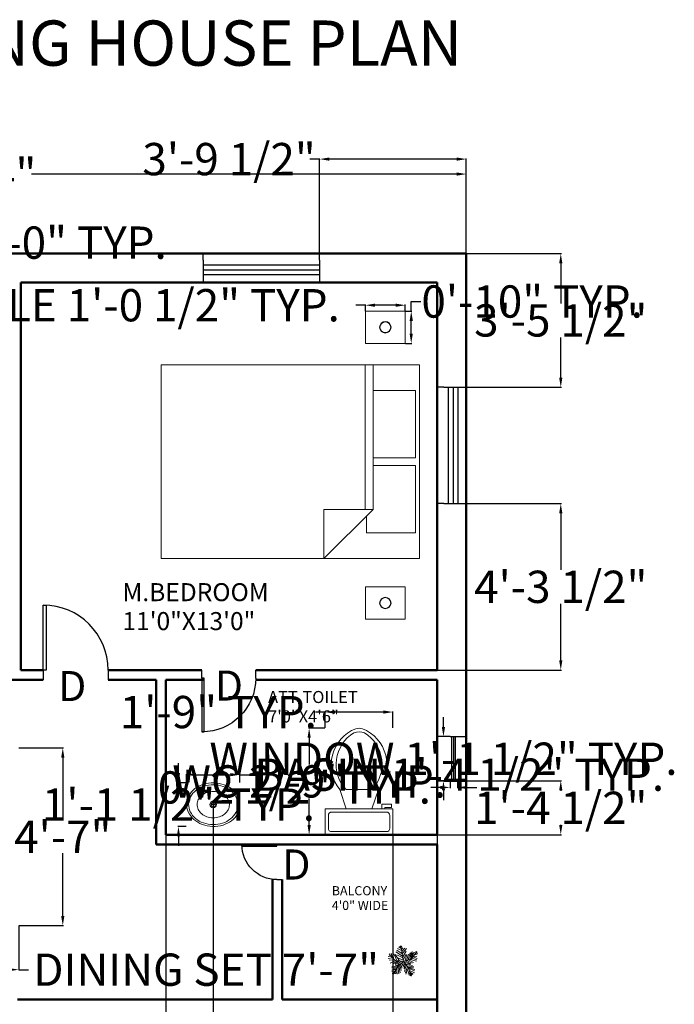
# Model space of a CAD drawing. Units: inches. Extents: x -35 to 382, y 867 to 1468.
# Tile 3 of 3: x 179 to 382, y 1163 to 1468. Entities that reach past the tile are written whole.
import ezdxf

# ---------------------------------------------------------------- set-up
doc = ezdxf.new("R2010")
doc.units = ezdxf.units.IN
doc.header["$MEASUREMENT"] = 0
for name, color, linetype, lineweight in [('A-ANNO-DIMS', 2, 'Continuous', 18), ('A-ANNO-TEXT', 7, 'Continuous', 25), ('A-AREA-IDEN', 7, 'Continuous', 25), ('A-DOOR', 3, 'Continuous', 25), ('A-FLOR-FIXT', 9, 'Continuous', 18), ('A-FURN', 9, 'Continuous', 18), ('A-GLAZ', 4, 'Continuous', 25), ('A-WALL', 7, 'Continuous', 50), ('L-PLNT', 94, 'Continuous', 13)]:
    doc.layers.add(name, color=color, linetype=linetype, lineweight=lineweight)
doc.styles.get("Standard").update_dxf_attribs({"font": 'arial.ttf'})
doc.dimstyles.get("Standard").update_dxf_attribs({"dimtxt": 10, "dimasz": 3, "dimexe": 0.18, "dimexo": 0.0625, "dimgap": 0.09, "dimtad": 0, "dimtih": 1, "dimtoh": 1, "dimdec": 0, "dimzin": 0, "dimdsep": 46, "dimlunit": 3, "dimtxsty": 'Standard', "dimcen": 0.09, "dimadec": 0, "dimazin": 0, "dimtfac": 1, "dimtdec": 0, "dimtofl": 0, "dimtmove": 0, "dimatfit": 3, "dimfxl": 1, "dimtolj": 1, "dimtzin": 0, "dimarcsym": 0})

# ---------------------------------------------------------------- blocks, each defined once
blk = doc.blocks.new('Bed - Queen')
for p, q in [((0, -80.00003), (0, 0)), ((0, 0), (59.99999, 0)), ((59.99999, 0), (59.99999, -80.00003)), ((7.99999, -1.2), (28.79998, -1.2)), ((7.99999, -14.4), (7.99999, -1.2)), ((28.79998, -1.2), (28.79998, -14.4)), ((31.19999, -1.2), (51.99999, -1.2)), ((31.19999, -14.4), (31.19999, -1.2)), ((51.99999, -1.2), (51.99999, -16.4)), ((0, -14.4), (44.8, -14.4)), ((59.99999, -29.6), (44.8, -14.4)), ((44.8, -14.4), (44.8, -29.6)), ((44.8, -16.8), (0, -16.8)), ((51.99999, -16.4), (46.79936, -16.4)), ((44.8, -29.6), (59.99999, -29.6)), ((59.99999, -80.00003), (0, -80.00003))]:
    blk.add_line(p, q)
blk = doc.blocks.new('Sink - Oval top')
for p, q in [((-1, 0), (1, 0)), ((0, 1), (0, -1))]:
    blk.add_line(p, q)
for points in [[(-12.23, 0.39, 0.117634), (-11.46, -3.36, 0.104469), (-8.88, -6.8, 0.090016), (-5.08, -9.07, 0.08192), (-0.32, -10.02, 0.08192), (4.49, -9.38, 0.090016), (8.42, -7.36, 0.104469), (11.22, -4.09, 0.117634), (12.23, -0.39, 0.117634), (11.46, 3.36, 0.104469), (8.88, 6.8, 0.090016), (5.08, 9.07, 0.08192), (0.32, 10.02, 0.08192), (-4.49, 9.38, 0.090016), (-8.42, 7.36, 0.104469), (-11.22, 4.09, 0.117634)], [(-11.29, 0.16, 0.118622), (-10.52, -3.25, 0.104678), (-8.07, -6.36, 0.089562), (-4.54, -8.37, 0.081185), (-0.13, -9.15, 0.081185), (4.3, -8.49, 0.089562), (7.89, -6.58, 0.104678), (10.42, -3.55, 0.118622), (11.29, -0.16, 0.118622), (10.52, 3.25, 0.104678), (8.07, 6.36, 0.089562), (4.54, 8.37, 0.081185), (0.13, 9.15, 0.081185), (-4.3, 8.49, 0.089562), (-7.89, 6.58, 0.104678), (-10.42, 3.55, 0.118622)], [(-7.42, 0.08, 0.118283), (-6.91, -2.17, 0.104607), (-5.29, -4.21, 0.089718), (-2.97, -5.53, 0.081436), (-0.07, -6.04, 0.081436), (2.84, -5.59, 0.089718), (5.2, -4.33, 0.104607), (6.86, -2.32, 0.118283), (7.42, -0.08, 0.118283), (6.91, 2.17, 0.104607), (5.29, 4.21, 0.089718), (2.97, 5.53, 0.081436), (0.07, 6.04, 0.081436), (-2.84, 5.59, 0.089718), (-5.2, 4.33, 0.104607), (-6.86, 2.32, 0.118283)]]:
    blk.add_lwpolyline(points, format="xyb", close=True)
for radius in [1.5, 1]:
    blk.add_circle((0, 0), radius)
blk = doc.blocks.new('*U13')
for p, q in [((-93.091, 489.5342), (-700.3796, 902.3858)), ((-129.8956, 713.6638), (-626.7704, 1032.1544)), ((-185.1152, 1008.5578), (-553.1612, 1185.4942)), ((-221.9198, 1197.3052), (-433.5526, 1338.8594)), ((-258.7244, 1362.456), (-332.3336, 1421.4348)), ((0, 0), (-266.7, 1447.8)), ((-231.1146, 1315.2628), (-166.7002, 1421.4348)), ((-194.31, 1102.9442), (-65.4812, 1256.284)), ((-148.3106, 914.1968), (118.5418, 1220.9018)), ((-129.8956, 701.8528), (265.7602, 1185.4942)), ((-74.7014, 418.7444), (219.7608, 961.39)), ((685.8, 228.6), (1219.2, 914.4)), ((689.0258, 230.0224), (790.2448, 914.1968)), ((1121.4862, 925.9824), (1149.0706, 831.6214)), ((-1206.4492, 501.3198), (-1418.082, 465.9376)), ((-1031.621, 347.98), (-1399.667, 277.1902)), ((-800.1, 114.3), (-1333.5, 647.7)), ((-847.598, 159.2326), (-1326.0578, 135.636)), ((-1234.059, 536.7274), (-1252.4486, 737.2604)), ((-718.7946, 88.4682), (-1215.644, -147.447)), ((-1105.2302, 725.4494), (-1077.6458, 395.1732)), ((-976.4268, 666.4706), (-884.4026, 194.6402)), ((-543.9664, 76.6572), (-967.2066, -206.4512)), ((-902.8176, 713.6638), (-617.5756, 100.2538)), ((0, 0), (-800.1, 114.3)), ((-369.1382, 53.086), (-783.1836, 642.874)), ((-405.9428, 53.086), (-764.794, -241.8334)), ((-617.5756, 607.4918), (-74.7014, 347.98)), ((0, 0), (-571.5, -495.3)), ((-166.7002, 29.4894), (-543.9664, -206.4512)), ((-525.5514, 347.98), (-28.6766, 123.8504)), ((-28.6766, 171.0436), (228.9556, 678.2816)), ((0, 0), (685.8, 228.6)), ((0, 0), (457.2, -571.5)), ((100.1268, 41.275), (284.1498, 619.2774)), ((164.5412, 41.275), (661.416, -218.2368)), ((256.5654, 88.4682), (449.7832, 666.4706)), ((284.1498, 88.4682), (781.0246, -147.447)), ((412.9786, 147.447), (587.8068, 796.2392)), ((458.978, 147.447), (891.4384, -88.4682)), ((560.197, 182.8292), (698.2206, 819.8358)), ((615.4166, 194.6402), (1185.8752, 41.275)), ((753.4148, 312.5978), (1222.6798, 159.2326)), ((808.6344, 784.4282), (827.0494, 418.7444)), ((845.439, 418.7444), (1241.0948, 277.1902)), ((891.4384, 831.6214), (946.658, 572.1096)), ((919.0482, 501.3198), (1222.6798, 454.152)), ((983.4626, 867.0036), (1066.2666, 725.4494)), ((1029.462, 654.685), (1241.0948, 631.0884)), ((1112.2914, 760.8316), (1296.3144, 784.4282)), ((-442.7474, -383.3876), (-1086.8406, -477.7486)), ((-718.7946, -737.2604), (-1086.8406, -796.2392)), ((-617.5756, -548.5384), (-1077.6458, -560.324)), ((-783.1836, -867.029), (-1077.6458, -902.4112)), ((-681.9646, -666.496), (-1022.4262, -654.685)), ((-571.5, -495.3), (-952.5, -1143)), ((-387.5278, -324.4088), (-764.794, -324.4088)), ((-737.1842, -784.4536), (-709.5744, -1114.7298)), ((-635.9652, -607.5172), (-580.771, -1150.1374)), ((-525.5514, -465.963), (-451.9422, -1126.5408)), ((-166.7002, -147.447), (-507.1618, -253.619)), ((-433.5526, -383.3876), (-323.1134, -1020.3688)), ((-341.5284, -289.0012), (-221.9198, -831.6214)), ((-240.3094, -218.2368), (-157.5054, -595.7062)), ((-120.7008, -88.4682), (-93.091, -371.5766)), ((63.3222, -76.6826), (-37.8714, -513.1308)), ((44.9326, -64.897), (615.4166, -241.8334)), ((127.7366, -159.258), (54.1274, -654.685)), ((228.9556, -289.0012), (90.932, -914.1968)), ((357.759, -430.5554), (164.5412, -1020.3688)), ((192.151, -230.0224), (817.8292, -371.5766)), ((458.978, -572.1096), (210.5406, -1161.923)), ((311.7596, -383.3876), (937.4378, -477.7486)), ((514.1976, -772.6426), (403.7838, -1138.3264)), ((412.9786, -501.3452), (919.0482, -583.9206)), ((457.2, -571.5), (685.8, -1333.5)), ((468.1982, -572.1096), (1029.462, -737.2604)), ((486.5878, -642.8994), (983.4626, -843.4324)), ((541.8074, -831.6214), (992.6574, -1032.1544)), ((-875.2078, -1008.5832), (-1040.8412, -1079.3476)), ((-829.2084, -937.7934), (-810.7934, -1126.5408)), ((578.612, -961.39), (495.7826, -1232.7128)), ((578.612, -973.1756), (873.0488, -1138.3264)), ((624.6114, -1161.923), (587.8068, -1291.6916)), ((624.6114, -1102.9442), (781.0246, -1209.1162)), ((679.8056, -1268.095), (716.6102, -1291.6916))]:
    blk.add_line(p, q)
blk = doc.blocks.new('*U9')
for p, q in [((0, 0), (0, -6)), ((40, 0), (40, -6))]:
    blk.add_line(p, q)
blk.add_lwpolyline([(0, 0), (0, 40), (1.75, 40), (1.75, 0)], close=True)
blk.add_arc((0, 0), 40, 0, 90)
blk = doc.blocks.new('Toilet - top')
for p, q in [((9.5, -6), (9.5, -2)), ((-10, -8.5), (-8, -8.5)), ((-10, -9.5), (-10, -8.5)), ((-8, -8.5), (-8, -8)), ((-7, -8), (-7, -9.5)), ((-4, -8), (-6, -14)), ((4, -8), (6, -14)), ((-7, -9.5), (-10, -9.5)), ((4, -14), (-4, -14))]:
    blk.add_line(p, q)
blk.add_lwpolyline([(10.5, -8), (10.5, 0), (-10.5, 0), (-10.5, -8)], close=True)
for points in [[(-9.5, -2), (-9.5, -6)], [(8.5, -1), (-8.5, -1)], [(-8.5, -7), (8.5, -7)]]:
    blk.add_lwpolyline(points)
for centre, radius, start, end in [((-8.62, -1.88), 0.884, 81.8699, 188.1301), ((8.62, -1.88), 0.884, 351.8699, 98.1301), ((-8.62, -6.12), 0.884, 171.8699, 278.1301), ((8.62, -6.12), 0.884, 261.8699, 8.1301), ((3.52, -21.58), 12.17, 141.4691, 247.9714), ((4.2, -21.82), 11.33, 136.3677, 238.9468), ((-3.52, -21.58), 12.17, 292.0284, 38.5307), ((-4.2, -21.82), 11.33, 301.053, 43.6321), ((0, -27.88), 4, 245.7318, 294.2682), ((0, -29), 4, 254.8605, 285.1395)]:
    blk.add_arc(centre, radius, start, end)
blk = doc.blocks.new('Window - Wood Frame 36 in. Wide plan')
for p, q in [((0, 6), (0, 0)), ((0, 4.5), (36, 4.5)), ((36, 6), (36, 0)), ((0, 3), (36, 3)), ((0, 1.5), (36, 1.5))]:
    blk.add_line(p, q)
blk = doc.blocks.new('*D15')
at = {"layer": 'A-ANNO-DIMS', "color": 0, "lineweight": -2, "transparency": 16777216}
for p, q in [((13.52, 1395.38), (13.52, 1420.11)), ((16.52, 1419.93), (148.17, 1419.93)), ((314.52, 1419.93), (182.87, 1419.93)), ((317.52, 1395.38), (317.52, 1420.11))]:
    blk.add_line(p, q, dxfattribs=at)
at = {"layer": 'A-ANNO-DIMS', "color": 0, "transparency": 16777216}
for points in [[(16.52, 1420.43), (16.52, 1419.43), (13.52, 1419.93)], [(314.52, 1420.43), (314.52, 1419.43), (317.52, 1419.93)]]:
    blk.add_solid(points, dxfattribs=at)
at = {"layer": 'Defpoints', "color": 0, "transparency": 16777216}
for p in [(317.52, 1419.93), (13.52, 1395.31), (317.52, 1395.31)]:
    blk.add_point(p, dxfattribs=at)
at = {"layer": 'A-ANNO-DIMS', "color": 0, "transparency": 16777216, "insert": (165.52, 1419.93), "char_height": 10, "attachment_point": 5}
blk.add_mtext('\\A1;25\'-4"', dxfattribs=at)
blk = doc.blocks.new('BEDSIDE-TABLE')
blk.add_lwpolyline([(0, 12.34), (9.96, 12.34), (9.96, 0), (0, 0)], close=True)
for radius in [1.78, 1.78, 1.66]:
    blk.add_circle((4.98, 6.17), radius)
blk = doc.blocks.new('*D18')
at = {"layer": 'A-ANNO-DIMS', "color": 0, "lineweight": -2, "transparency": 16777216}
for p, q in [((61.69, 1393.35), (61.69, 1398.87)), ((64.69, 1398.69), (94.69, 1398.69)), ((97.69, 1393.35), (97.69, 1398.87)), ((97.69, 1398.69), (100.69, 1398.69))]:
    blk.add_line(p, q, dxfattribs=at)
at = {"layer": 'A-ANNO-DIMS', "color": 0, "transparency": 16777216}
for points in [[(64.69, 1399.19), (64.69, 1398.19), (61.69, 1398.69)], [(94.69, 1399.19), (94.69, 1398.19), (97.69, 1398.69)]]:
    blk.add_solid(points, dxfattribs=at)
at = {"layer": 'Defpoints', "color": 0, "transparency": 16777216}
for p in [(97.69, 1398.69), (61.69, 1393.29), (97.69, 1393.29)]:
    blk.add_point(p, dxfattribs=at)
at = {"layer": 'A-ANNO-DIMS', "color": 0, "transparency": 16777216, "insert": (164.05, 1398.69), "char_height": 10, "attachment_point": 5}
blk.add_mtext('\\A1;WINDOW 3\'-0" TYP.', dxfattribs=at)
blk = doc.blocks.new('*D20')
at = {"layer": 'A-ANNO-DIMS', "color": 0, "lineweight": -2, "transparency": 16777216}
for p, q in [((310.44, 1248.71), (310.44, 1251.71)), ((312.43, 1245.71), (310.26, 1245.71)), ((312.43, 1232.03), (310.26, 1232.03)), ((310.44, 1229.03), (310.44, 1226.03))]:
    blk.add_line(p, q, dxfattribs=at)
at = {"layer": 'A-ANNO-DIMS', "color": 0, "transparency": 16777216}
for points in [[(309.94, 1248.71), (310.94, 1248.71), (310.44, 1245.71)], [(309.94, 1229.03), (310.94, 1229.03), (310.44, 1232.03)]]:
    blk.add_solid(points, dxfattribs=at)
at = {"layer": 'Defpoints', "color": 0, "transparency": 16777216}
for p in [(310.44, 1245.71), (312.49, 1245.71), (312.49, 1232.03)]:
    blk.add_point(p, dxfattribs=at)
at = {"layer": 'A-ANNO-DIMS', "color": 0, "transparency": 16777216, "insert": (310.44, 1238.87), "char_height": 10, "attachment_point": 5}
blk.add_mtext('\\A1;WINDOW 1\'-1 1/2" TYP.', dxfattribs=at)
blk = doc.blocks.new('*D21')
at = {"layer": 'A-ANNO-DIMS', "color": 0, "lineweight": -2, "transparency": 16777216}
for p, q in [((312.49, 1231.96), (312.49, 1229.79)), ((314.77, 1231.96), (314.77, 1229.79)), ((309.49, 1229.97), (306.49, 1229.97)), ((317.77, 1229.97), (320.77, 1229.97))]:
    blk.add_line(p, q, dxfattribs=at)
at = {"layer": 'A-ANNO-DIMS', "color": 0, "transparency": 16777216}
for points in [[(309.49, 1230.47), (309.49, 1229.47), (312.49, 1229.97)], [(317.77, 1230.47), (317.77, 1229.47), (314.77, 1229.97)]]:
    blk.add_solid(points, dxfattribs=at)
at = {"layer": 'Defpoints', "color": 0, "transparency": 16777216}
for p in [(312.49, 1232.03), (314.77, 1232.03), (312.49, 1229.97)]:
    blk.add_point(p, dxfattribs=at)
at = {"layer": 'A-ANNO-DIMS', "color": 0, "transparency": 16777216, "insert": (264.27, 1229.97), "char_height": 10, "attachment_point": 5}
blk.add_mtext('\\A1;0\'-2 1/2" TYP.', dxfattribs=at)
blk = doc.blocks.new('*D22')
at = {"layer": 'A-ANNO-DIMS', "color": 0, "lineweight": -2, "transparency": 16777216}
for p, q in [((286.27, 1379.31), (283.27, 1379.31)), ((286.27, 1377.52), (286.27, 1379.49)), ((295.61, 1379.31), (289.27, 1379.31)), ((298.61, 1377.52), (298.61, 1379.49))]:
    blk.add_line(p, q, dxfattribs=at)
at = {"layer": 'A-ANNO-DIMS', "color": 0, "transparency": 16777216}
for points in [[(289.27, 1379.81), (289.27, 1378.81), (286.27, 1379.31)], [(295.61, 1379.81), (295.61, 1378.81), (298.61, 1379.31)]]:
    blk.add_solid(points, dxfattribs=at)
at = {"layer": 'Defpoints', "color": 0, "transparency": 16777216}
for p in [(286.27, 1379.31), (286.27, 1377.46), (298.61, 1377.46)]:
    blk.add_point(p, dxfattribs=at)
at = {"layer": 'A-ANNO-DIMS', "color": 0, "transparency": 16777216, "insert": (184.6, 1379.31), "char_height": 10, "attachment_point": 5}
blk.add_mtext('\\A1;BEDSIDE TABLE 1\'-0 1/2" TYP.', dxfattribs=at)
blk = doc.blocks.new('*D23')
at = {"layer": 'A-ANNO-DIMS', "color": 0, "lineweight": -2, "transparency": 16777216}
for p, q in [((300.46, 1377.46), (300.46, 1380.46)), ((300.46, 1380.46), (303.46, 1380.46)), ((298.67, 1377.46), (300.64, 1377.46)), ((300.46, 1370.5), (300.46, 1374.46)), ((298.67, 1367.5), (300.64, 1367.5))]:
    blk.add_line(p, q, dxfattribs=at)
at = {"layer": 'A-ANNO-DIMS', "color": 0, "transparency": 16777216}
for points in [[(299.96, 1374.46), (300.96, 1374.46), (300.46, 1377.46)], [(299.96, 1370.5), (300.96, 1370.5), (300.46, 1367.5)]]:
    blk.add_solid(points, dxfattribs=at)
at = {"layer": 'Defpoints', "color": 0, "transparency": 16777216}
for p in [(298.61, 1377.46), (300.46, 1377.46), (298.61, 1367.5)]:
    blk.add_point(p, dxfattribs=at)
at = {"layer": 'A-ANNO-DIMS', "color": 0, "transparency": 16777216, "insert": (337.91, 1380.46), "char_height": 10, "attachment_point": 5}
blk.add_mtext('\\A1;0\'-10" TYP.', dxfattribs=at)
blk = doc.blocks.new('*D26')
at = {"layer": 'A-ANNO-DIMS', "color": 0, "lineweight": -2, "transparency": 16777216}
for p, q in [((230.86, 1231.51), (230.86, 1234.11)), ((233.86, 1233.93), (244.43, 1233.93)), ((247.43, 1231.51), (247.43, 1234.11)), ((247.43, 1233.93), (250.43, 1233.93))]:
    blk.add_line(p, q, dxfattribs=at)
at = {"layer": 'A-ANNO-DIMS', "color": 0, "transparency": 16777216}
for points in [[(233.86, 1234.43), (233.86, 1233.43), (230.86, 1233.93)], [(244.43, 1234.43), (244.43, 1233.43), (247.43, 1233.93)]]:
    blk.add_solid(points, dxfattribs=at)
at = {"layer": 'Defpoints', "color": 0, "transparency": 16777216}
for p in [(247.43, 1233.93), (230.86, 1231.45), (247.43, 1231.45)]:
    blk.add_point(p, dxfattribs=at)
at = {"layer": 'A-ANNO-DIMS', "color": 0, "transparency": 16777216, "insert": (315.33, 1233.93), "char_height": 10, "attachment_point": 5}
blk.add_mtext('\\A1;BASIN 1\'-4 1/2" TYP.', dxfattribs=at)
blk = doc.blocks.new('*D27')
at = {"layer": 'A-ANNO-DIMS', "color": 0, "lineweight": -2, "transparency": 16777216}
for p, q in [((228.38, 1234.45), (228.38, 1237.45)), ((230.8, 1231.45), (228.2, 1231.45)), ((230.8, 1217.86), (228.2, 1217.86)), ((228.38, 1214.86), (228.38, 1211.86))]:
    blk.add_line(p, q, dxfattribs=at)
at = {"layer": 'A-ANNO-DIMS', "color": 0, "transparency": 16777216}
for points in [[(227.88, 1234.45), (228.88, 1234.45), (228.38, 1231.45)], [(227.88, 1214.86), (228.88, 1214.86), (228.38, 1217.86)]]:
    blk.add_solid(points, dxfattribs=at)
at = {"layer": 'Defpoints', "color": 0, "transparency": 16777216}
for p in [(228.38, 1231.45), (230.86, 1231.45), (230.86, 1217.86)]:
    blk.add_point(p, dxfattribs=at)
at = {"layer": 'A-ANNO-DIMS', "color": 0, "transparency": 16777216, "insert": (228.38, 1224.65), "char_height": 10, "attachment_point": 5}
blk.add_mtext('\\A1;1\'-1 1/2" TYP.', dxfattribs=at)
blk = doc.blocks.new('*D28')
at = {"layer": 'A-ANNO-DIMS', "color": 0, "lineweight": -2, "transparency": 16777216}
for p, q in [((273.75, 1248.36), (268.67, 1248.36)), ((268.85, 1245.36), (268.85, 1237.1)), ((268.85, 1218.31), (268.85, 1226.58)), ((273.75, 1215.31), (268.67, 1215.31))]:
    blk.add_line(p, q, dxfattribs=at)
at = {"layer": 'A-ANNO-DIMS', "color": 0, "transparency": 16777216}
for points in [[(268.35, 1245.36), (269.35, 1245.36), (268.85, 1248.36)], [(268.35, 1218.31), (269.35, 1218.31), (268.85, 1215.31)]]:
    blk.add_solid(points, dxfattribs=at)
at = {"layer": 'Defpoints', "color": 0, "transparency": 16777216}
for p in [(273.81, 1248.36), (268.85, 1215.31), (273.81, 1215.31)]:
    blk.add_point(p, dxfattribs=at)
at = {"layer": 'A-ANNO-DIMS', "color": 0, "transparency": 16777216, "insert": (268.85, 1231.84), "char_height": 10, "attachment_point": 5}
blk.add_mtext('\\A1;WC 2\'-9" TYP.', dxfattribs=at)
blk = doc.blocks.new('*D29')
at = {"layer": 'A-ANNO-DIMS', "color": 0, "lineweight": -2, "transparency": 16777216}
for p, q in [((273.81, 1253.32), (270.81, 1253.32)), ((273.81, 1248.42), (273.81, 1253.5)), ((291.81, 1253.32), (276.81, 1253.32)), ((294.81, 1248.42), (294.81, 1253.5))]:
    blk.add_line(p, q, dxfattribs=at)
at = {"layer": 'A-ANNO-DIMS', "color": 0, "transparency": 16777216}
for points in [[(276.81, 1253.82), (276.81, 1252.82), (273.81, 1253.32)], [(291.81, 1253.82), (291.81, 1252.82), (294.81, 1253.32)]]:
    blk.add_solid(points, dxfattribs=at)
at = {"layer": 'Defpoints', "color": 0, "transparency": 16777216}
for p in [(273.81, 1253.32), (273.81, 1248.36), (294.81, 1248.36)]:
    blk.add_point(p, dxfattribs=at)
at = {"layer": 'A-ANNO-DIMS', "color": 0, "transparency": 16777216, "insert": (240.72, 1253.32), "char_height": 10, "attachment_point": 5}
blk.add_mtext('\\A1;1\'-9" TYP.', dxfattribs=at)
blk = doc.blocks.new('*D36')
at = {"layer": 'A-ANNO-DIMS', "color": 0, "lineweight": -2, "transparency": 16777216}
for p, q in [((87.91, 1187.13), (87.91, 1173.36)), ((178.91, 1187.13), (178.91, 1173.36)), ((90.91, 1173.54), (175.91, 1173.54)), ((178.91, 1173.54), (181.91, 1173.54))]:
    blk.add_line(p, q, dxfattribs=at)
at = {"layer": 'A-ANNO-DIMS', "color": 0, "transparency": 16777216}
for points in [[(90.91, 1174.04), (90.91, 1173.04), (87.91, 1173.54)], [(175.91, 1174.04), (175.91, 1173.04), (178.91, 1173.54)]]:
    blk.add_solid(points, dxfattribs=at)
at = {"layer": 'Defpoints', "color": 0, "transparency": 16777216}
for p in [(87.91, 1187.19), (178.91, 1187.19), (178.91, 1173.54)]:
    blk.add_point(p, dxfattribs=at)
at = {"layer": 'A-ANNO-DIMS', "color": 0, "transparency": 16777216, "insert": (236.96, 1173.54), "char_height": 10, "attachment_point": 5}
blk.add_mtext('\\A1;DINING SET 7\'-7"', dxfattribs=at)
blk = doc.blocks.new('*D37')
at = {"layer": 'A-ANNO-DIMS', "color": 0, "lineweight": -2, "transparency": 16777216}
for p, q in [((178.97, 1242.19), (192.74, 1242.19)), ((192.56, 1239.19), (192.56, 1219.78)), ((192.56, 1190.19), (192.56, 1209.6)), ((178.97, 1187.19), (192.74, 1187.19))]:
    blk.add_line(p, q, dxfattribs=at)
at = {"layer": 'A-ANNO-DIMS', "color": 0, "transparency": 16777216}
for points in [[(192.06, 1239.19), (193.06, 1239.19), (192.56, 1242.19)], [(192.06, 1190.19), (193.06, 1190.19), (192.56, 1187.19)]]:
    blk.add_solid(points, dxfattribs=at)
at = {"layer": 'Defpoints', "color": 0, "transparency": 16777216}
for p in [(178.91, 1242.19), (192.56, 1242.19), (178.91, 1187.19)]:
    blk.add_point(p, dxfattribs=at)
at = {"layer": 'A-ANNO-DIMS', "color": 0, "transparency": 16777216, "insert": (192.56, 1214.69), "char_height": 10, "attachment_point": 5}
blk.add_mtext('\\A1;4\'-7"', dxfattribs=at)
blk = doc.blocks.new('*D43')
at = {"layer": 'A-ANNO-DIMS', "color": 0, "lineweight": -2, "transparency": 16777216}
for p, q in [((317.58, 1317.89), (346.95, 1317.89)), ((346.77, 1314.89), (346.77, 1297.36)), ((346.77, 1269.31), (346.77, 1286.84)), ((308.58, 1266.31), (346.95, 1266.31))]:
    blk.add_line(p, q, dxfattribs=at)
at = {"layer": 'A-ANNO-DIMS', "color": 0, "transparency": 16777216}
for points in [[(346.27, 1314.89), (347.27, 1314.89), (346.77, 1317.89)], [(346.27, 1269.31), (347.27, 1269.31), (346.77, 1266.31)]]:
    blk.add_solid(points, dxfattribs=at)
at = {"layer": 'Defpoints', "color": 0, "transparency": 16777216}
for p in [(317.52, 1317.89), (308.52, 1266.31), (346.77, 1266.31)]:
    blk.add_point(p, dxfattribs=at)
at = {"layer": 'A-ANNO-DIMS', "color": 0, "transparency": 16777216, "insert": (346.77, 1292.1), "char_height": 10, "attachment_point": 5}
blk.add_mtext('\\A1;4\'-3 1/2"', dxfattribs=at)
blk = doc.blocks.new('*D45')
at = {"layer": 'A-ANNO-DIMS', "color": 0, "lineweight": -2, "transparency": 16777216}
for p, q in [((239.15, 1224.59), (239.15, 881.88)), ((224.52, 1215.25), (224.52, 881.88)), ((227.52, 882.06), (236.15, 882.06)), ((239.15, 882.06), (242.15, 882.06))]:
    blk.add_line(p, q, dxfattribs=at)
at = {"layer": 'A-ANNO-DIMS', "color": 0, "transparency": 16777216}
for points in [[(227.52, 882.56), (227.52, 881.56), (224.52, 882.06)], [(236.15, 882.56), (236.15, 881.56), (239.15, 882.06)]]:
    blk.add_solid(points, dxfattribs=at)
at = {"layer": 'Defpoints', "color": 0, "transparency": 16777216}
for p in [(239.15, 1224.65), (224.52, 1215.31), (239.15, 882.06)]:
    blk.add_point(p, dxfattribs=at)
at = {"layer": 'A-ANNO-DIMS', "color": 0, "transparency": 16777216, "insert": (266.71, 882.06), "char_height": 10, "attachment_point": 5}
blk.add_mtext('\\A1;1\'-2 1/2"', dxfattribs=at)
blk = doc.blocks.new('*D46')
at = {"layer": 'A-ANNO-DIMS', "color": 0, "lineweight": -2, "transparency": 16777216}
for p, q in [((294.81, 1215.25), (294.81, 881.88)), ((308.52, 1215.25), (308.52, 881.88)), ((294.81, 882.06), (291.81, 882.06)), ((305.52, 882.06), (297.81, 882.06))]:
    blk.add_line(p, q, dxfattribs=at)
at = {"layer": 'A-ANNO-DIMS', "color": 0, "transparency": 16777216}
for points in [[(297.81, 882.56), (297.81, 881.56), (294.81, 882.06)], [(305.52, 882.56), (305.52, 881.56), (308.52, 882.06)]]:
    blk.add_solid(points, dxfattribs=at)
at = {"layer": 'Defpoints', "color": 0, "transparency": 16777216}
for p in [(294.81, 1215.31), (308.52, 1215.31), (294.81, 882.06)]:
    blk.add_point(p, dxfattribs=at)
at = {"layer": 'A-ANNO-DIMS', "color": 0, "transparency": 16777216, "insert": (267.25, 882.06), "char_height": 10, "attachment_point": 5}
blk.add_mtext('\\A1;1\'-1 1/2"', dxfattribs=at)
blk = doc.blocks.new('*D48')
at = {"layer": 'A-ANNO-DIMS', "color": 0, "lineweight": -2, "transparency": 16777216}
for p, q in [((272.07, 1424.56), (269.07, 1424.56)), ((272.07, 1395.38), (272.07, 1424.74)), ((314.52, 1424.56), (275.07, 1424.56)), ((317.52, 1395.38), (317.52, 1424.74))]:
    blk.add_line(p, q, dxfattribs=at)
at = {"layer": 'A-ANNO-DIMS', "color": 0, "transparency": 16777216}
for points in [[(275.07, 1425.06), (275.07, 1424.06), (272.07, 1424.56)], [(314.52, 1425.06), (314.52, 1424.06), (317.52, 1424.56)]]:
    blk.add_solid(points, dxfattribs=at)
at = {"layer": 'Defpoints', "color": 0, "transparency": 16777216}
for p in [(272.07, 1424.56), (272.07, 1395.31), (317.52, 1395.31)]:
    blk.add_point(p, dxfattribs=at)
at = {"layer": 'A-ANNO-DIMS', "color": 0, "transparency": 16777216, "insert": (244.04, 1424.56), "char_height": 10, "attachment_point": 5}
blk.add_mtext('\\A1;3\'-9 1/2"', dxfattribs=at)
blk = doc.blocks.new('*D49')
at = {"layer": 'A-ANNO-DIMS', "color": 0, "lineweight": -2, "transparency": 16777216}
for p, q in [((317.58, 1395.31), (346.95, 1395.31)), ((346.77, 1392.31), (346.77, 1379.86)), ((346.77, 1356.89), (346.77, 1369.34)), ((317.58, 1353.89), (346.95, 1353.89))]:
    blk.add_line(p, q, dxfattribs=at)
at = {"layer": 'A-ANNO-DIMS', "color": 0, "transparency": 16777216}
for points in [[(346.27, 1392.31), (347.27, 1392.31), (346.77, 1395.31)], [(346.27, 1356.89), (347.27, 1356.89), (346.77, 1353.89)]]:
    blk.add_solid(points, dxfattribs=at)
at = {"layer": 'Defpoints', "color": 0, "transparency": 16777216}
for p in [(317.52, 1395.31), (317.52, 1353.89), (346.77, 1353.89)]:
    blk.add_point(p, dxfattribs=at)
at = {"layer": 'A-ANNO-DIMS', "color": 0, "transparency": 16777216, "insert": (346.77, 1374.6), "char_height": 10, "attachment_point": 5}
blk.add_mtext('\\A1;3\'-5 1/2"', dxfattribs=at)
blk = doc.blocks.new('*D53')
at = {"layer": 'A-ANNO-DIMS', "color": 0, "lineweight": -2, "transparency": 16777216}
for p, q in [((308.58, 1232.03), (346.95, 1232.03)), ((346.77, 1229.03), (346.77, 1228.93)), ((346.77, 1218.31), (346.77, 1218.41)), ((308.58, 1215.31), (346.95, 1215.31))]:
    blk.add_line(p, q, dxfattribs=at)
at = {"layer": 'A-ANNO-DIMS', "color": 0, "transparency": 16777216}
for points in [[(346.27, 1229.03), (347.27, 1229.03), (346.77, 1232.03)], [(346.27, 1218.31), (347.27, 1218.31), (346.77, 1215.31)]]:
    blk.add_solid(points, dxfattribs=at)
at = {"layer": 'Defpoints', "color": 0, "transparency": 16777216}
for p in [(308.52, 1232.03), (346.77, 1232.03), (308.52, 1215.31)]:
    blk.add_point(p, dxfattribs=at)
at = {"layer": 'A-ANNO-DIMS', "color": 0, "transparency": 16777216, "insert": (346.77, 1223.67), "char_height": 10, "attachment_point": 5}
blk.add_mtext('\\A1;1\'-4 1/2"', dxfattribs=at)

msp = doc.modelspace()

# ---------------------------------------------------------------- linework, layer by layer
at = {"layer": 'A-GLAZ'}
for p, q in [((236.07, 1393.29), (236.07, 1395.31)), ((272.07, 1393.29), (272.07, 1395.31)), ((236.07, 1387.29), (236.07, 1386.31)), ((272.07, 1387.29), (272.07, 1386.31)), ((310.54, 1353.89), (308.52, 1353.89)), ((316.54, 1353.89), (317.52, 1353.89)), ((310.54, 1317.89), (308.52, 1317.89)), ((316.54, 1317.89), (317.52, 1317.89)), ((311.72, 1245.71), (308.52, 1245.71)), ((312.49, 1245.71), (311.72, 1245.71)), ((314.77, 1245.71), (315.14, 1245.71)), ((315.14, 1245.71), (317.52, 1245.71)), ((311.72, 1232.03), (308.52, 1232.03)), ((312.49, 1232.03), (311.72, 1232.03)), ((314.77, 1232.03), (315.14, 1232.03)), ((315.14, 1232.03), (317.52, 1232.03))]:
    msp.add_line(p, q, dxfattribs=at)
at = {"layer": 'A-WALL'}
for p, q in [((13.52, 1395.31), (317.52, 1395.31)), ((317.52, 1098.31), (317.52, 1395.31)), ((317.52, 911.31), (317.52, 1395.31)), ((179.52, 1266.31), (179.52, 1386.31)), ((179.52, 1386.31), (308.52, 1386.31)), ((308.52, 1266.31), (308.52, 1386.31)), ((308.52, 1266.31), (308.52, 1386.31)), ((179.52, 1266.31), (186.49, 1266.31)), ((206.6, 1266.31), (235.66, 1266.31)), ((252.32, 1266.31), (308.52, 1266.31)), ((176.52, 1263.31), (186.49, 1263.31)), ((206.6, 1263.31), (221.52, 1263.31)), ((221.52, 1212.31), (221.52, 1263.31)), ((224.52, 1215.31), (224.52, 1263.31)), ((224.52, 1263.31), (236.39, 1263.31)), ((252.31, 1263.31), (308.52, 1263.31)), ((308.52, 1215.31), (308.52, 1263.31)), ((308.52, 1215.31), (308.52, 1263.31)), ((224.52, 1215.31), (273.81, 1215.31)), ((271.39, 1215.31), (308.52, 1215.31)), ((221.52, 1212.31), (308.52, 1212.31)), ((257.52, 1211.84), (257.52, 1212.31)), ((260.52, 1212.31), (261, 1212.31)), ((271.3, 1212.31), (308.52, 1212.31)), ((308.52, 1098.31), (308.52, 1212.31)), ((308.52, 918.31), (308.52, 1212.31)), ((257.52, 1164.31), (257.52, 1201.53)), ((260.52, 1164.31), (260.52, 1201.45)), ((178.52, 1164.31), (257.52, 1164.31)), ((260.52, 1164.31), (308.52, 1164.31))]:
    msp.add_line(p, q, dxfattribs=at)

# ---------------------------------------------------------------- block references
at = {"layer": 'A-DOOR', "xscale": 0.502721447591137, "yscale": 0.502721447591137, "zscale": 0.502721447591137}
msp.add_blockref('*U9', (186.49, 1266.33), dxfattribs=at)
at = {"layer": 'A-DOOR'}
for p, xscale, yscale, zscale, rotation in [((235.66, 1263.82), -0.416421438962062, 0.416421438962062, 0.416421438962062, 180), ((258.89, 1212.31), -0.2717391304347826, 0.2717391304347826, 0.2717391304347826, 90)]:
    msp.add_blockref('*U9', p, dxfattribs=dict(at, xscale=xscale, yscale=yscale, zscale=zscale, rotation=rotation))
at = {"layer": 'A-FLOR-FIXT', "rotation": 180}
msp.add_blockref('Toilet - top', (284.31, 1215.31), dxfattribs=at)
at = {"layer": 'A-FLOR-FIXT', "xscale": 0.6747385210637662, "yscale": 0.6747385210637662, "zscale": 0.6747385210637662}
msp.add_blockref('Sink - Oval top', (239.15, 1224.65), dxfattribs=at)
at = {"layer": 'A-FURN'}
for name, p, rotation in [('BEDSIDE-TABLE', (298.61, 1367.5), 89.999999999999), ('Bed - Queen', (303.03, 1360.87), 270), ('BEDSIDE-TABLE', (298.61, 1282.11), 90.00000000000018)]:
    msp.add_blockref(name, p, dxfattribs=dict(at, rotation=rotation))
at = {"layer": 'A-GLAZ'}
msp.add_blockref('Window - Wood Frame 36 in. Wide plan', (236.07, 1387.29), dxfattribs=at)
at = {"layer": 'A-GLAZ', "rotation": 90}
msp.add_blockref('Window - Wood Frame 36 in. Wide plan', (316.54, 1317.89), dxfattribs=at)
at = {"layer": 'A-GLAZ', "xscale": 0.3799930958700458, "yscale": 0.3799930958700458, "zscale": 0.3799930958700458, "rotation": 90}
msp.add_blockref('Window - Wood Frame 36 in. Wide plan', (314.77, 1232.03), dxfattribs=at)
at = {"layer": 'L-PLNT', "xscale": 0.0033829355053961, "yscale": 0.0033829355053961, "zscale": 0.0033829355053961}
msp.add_blockref('*U13', (298.1, 1176.05), dxfattribs=at)

# ---------------------------------------------------------------- texts
at = {"layer": 'A-ANNO-TEXT'}
for s, height, p in [('2BHK NORTH FACING HOUSE PLAN', 14.0085, (4.86, 1453.48)), ('D', 9.31, (191.11, 1256.72)), ('D', 9.31, (239.63, 1256.87)), ('D', 9.31, (260.52, 1201.45))]:
    msp.add_text(s, height=height, dxfattribs=at).set_placement(p)
at = {"layer": 'A-AREA-IDEN'}
for s, height, p in [('M.BEDROOM', 5.578, (211.02, 1287.66)), ('11\'0"X13\'0"', 5.5777, (211.02, 1278.7)), ('ATT.TOILET', 3.734, (256.13, 1256.11)), ('7\'0"X4\'6"', 3.734, (256.13, 1250.11)), ('BALCONY', 2.828, (275.87, 1196.58)), ('4\'0" WIDE', 2.828, (275.87, 1192.03))]:
    msp.add_text(s, height=height, dxfattribs=at).set_placement(p)

# ---------------------------------------------------------------- dimensions: what is measured, and where the dimension line sits
at = {"layer": 'A-ANNO-DIMS'}
for base, p1, p2, override, picture, middle in [((272.0734, 1424.5649), (317.5213, 1395.3149), (272.0734, 1395.3149), {"dimdec": 1, "dimlfac": 1, "dimrnd": 0, "dimzin": 1, "dimdsep": 46, "dimlunit": 4, "dimfrac": 2}, '*D48', (244.0448, 1424.5649)), ((317.52, 1419.93), (13.52, 1395.31), (317.52, 1395.31), {"dimclrd": 0, "dimclre": 0, "dimclrt": 0}, '*D15', (165.52, 1419.93)), ((239.15, 882.06), (224.52, 1215.31), (239.15, 1224.65), {"dimdec": 1, "dimlfac": 1, "dimrnd": 0, "dimzin": 1, "dimdsep": 46, "dimlunit": 4, "dimfrac": 2}, '*D45', (266.71, 882.06)), ((294.81, 882.06), (308.52, 1215.31), (294.81, 1215.31), {"dimdec": 1, "dimlfac": 1, "dimrnd": 0, "dimzin": 1, "dimdsep": 46, "dimlunit": 4, "dimfrac": 2}, '*D46', (267.25, 882.06))]:
    dim = msp.add_linear_dim(base=base, p1=p1, p2=p2, dimstyle='Standard', override=override, dxfattribs=at)
    dim.commit()
    dim.dimension.update_dxf_attribs({"geometry": picture, "text_midpoint": middle})
for base, p1, p2, text, picture, middle in [((97.69, 1398.69), (61.69, 1393.29), (97.69, 1393.29), 'WINDOW <> TYP.', '*D18', (164.05, 1398.69)), ((247.43, 1233.93), (230.86, 1231.45), (247.43, 1231.45), 'BASIN <> TYP.', '*D26', (315.33, 1233.93)), ((178.91, 1173.54), (87.91, 1187.19), (178.91, 1187.19), 'DINING SET <>', '*D36', (236.96, 1173.54))]:
    dim = msp.add_linear_dim(base=base, p1=p1, p2=p2, text=text, dimstyle='Standard', override={"dimdec": 1, "dimlfac": 1, "dimrnd": 0, "dimzin": 1, "dimdsep": 46, "dimlunit": 4, "dimfrac": 2}, dxfattribs=at)
    dim.commit()
    dim.dimension.update_dxf_attribs({"geometry": picture, "text_midpoint": middle})
for base, p1, p2, angle, text, picture, middle in [((286.27, 1379.31), (298.61, 1377.46), (286.27, 1377.46), 180, 'BEDSIDE TABLE <> TYP.', '*D22', (184.6, 1379.31)), ((300.46, 1377.46), (298.61, 1367.5), (298.61, 1377.46), 90, '<> TYP.', '*D23', (337.91, 1380.46)), ((310.44, 1245.71), (312.49, 1232.03), (312.49, 1245.71), 90, 'WINDOW <> TYP.', '*D20', (310.44, 1238.87)), ((273.81, 1253.32), (294.81, 1248.36), (273.81, 1248.36), 180, '<> TYP.', '*D29', (240.72, 1253.32)), ((312.49, 1229.97), (314.77, 1232.03), (312.49, 1232.03), 180, '<> TYP.', '*D21', (264.27, 1229.97)), ((268.855, 1215.3149), (273.8119, 1248.3612), (273.8119, 1215.3149), 270, 'WC <> TYP.', '*D28', (268.855, 1231.838)), ((228.38, 1231.45), (230.86, 1217.86), (230.86, 1231.45), 90, '<> TYP.', '*D27', (228.38, 1224.65))]:
    dim = msp.add_linear_dim(base=base, p1=p1, p2=p2, angle=angle, text=text, dimstyle='Standard', override={"dimdec": 1, "dimlfac": 1, "dimrnd": 0, "dimzin": 1, "dimdsep": 46, "dimlunit": 4, "dimfrac": 2}, dxfattribs=at)
    dim.commit()
    dim.dimension.update_dxf_attribs({"geometry": picture, "text_midpoint": middle})
for base, p1, p2, picture, middle in [((346.77, 1353.89), (317.52, 1395.31), (317.52, 1353.89), '*D49', (346.77, 1374.6)), ((346.77, 1266.31), (317.52, 1317.89), (308.52, 1266.31), '*D43', (346.77, 1292.1)), ((192.56, 1242.19), (178.91, 1187.19), (178.91, 1242.19), '*D37', (192.56, 1214.69)), ((346.77, 1232.03), (308.52, 1215.31), (308.52, 1232.03), '*D53', (346.77, 1223.67))]:
    dim = msp.add_linear_dim(base=base, p1=p1, p2=p2, angle=90, dimstyle='Standard', override={"dimdec": 1, "dimlfac": 1, "dimrnd": 0, "dimzin": 1, "dimdsep": 46, "dimlunit": 4, "dimfrac": 2}, dxfattribs=at)
    dim.commit()
    dim.dimension.update_dxf_attribs({"geometry": picture, "text_midpoint": middle})

doc.saveas('drawing.dxf')
